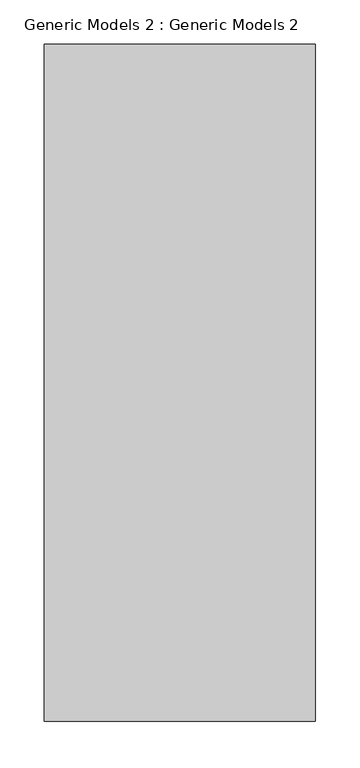
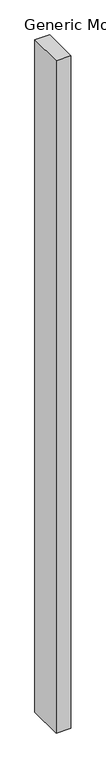
"""IFC4 building model written with IfcOpenShell, lengths in millimetres: proxy geometry, Generic Models 2 : Generic Models 2."""

from ifc_helpers import new_model, si_unit, frame, origin, place, context, project, spatial, polyline, outline, extrude, source, transform, mapped, element, save


def generic_models_2_generic_models_2_fd6437b6(model_context):
    return source(origin(), model_context, "Body", "SweptSolid", [
        extrude(outline(polyline([(13598.5361222, -384.9902311), (13598.5361222, 377.0097689), (13903.3361222, 377.0097689), (13903.3361222, -384.9902311), (13598.5361222, -384.9902311)])), frame((0.0, 0.0, 3840.2215532), z_axis=(0.0, 0.0, 1.0), x_axis=(1.0, 0.0, 0.0)), (0.0, 0.0, 1.0), 14782.8),
    ])


if __name__ == "__main__":
    model = new_model("IFC4")
    model_context = context("Model", 3, world=origin())
    ifc_project = project(units=[si_unit("LENGTHUNIT", "METRE", prefix="MILLI")], contexts=[model_context])
    site = spatial("IfcSite", under=ifc_project)
    building = spatial("IfcBuilding", under=site)
    placement = place(None, origin())
    generic_models_2_generic_models_2_shape = generic_models_2_generic_models_2_fd6437b6(model_context)
    element("IfcBuildingElementProxy", 1, Name="Generic Models 2 : Generic Models 2", ObjectType="Generic Models 2 : Generic Models 2", at=placement, inside=building, context=model_context, shape_type="MappedRepresentation", body=[
        mapped(generic_models_2_generic_models_2_shape, transform((0.0, 0.0, 0.0), x_axis=(1.0, 0.0, 0.0), y_axis=(0.0, 1.0, 0.0), z_axis=(0.0, 0.0, 1.0))),
    ])
    save(model, "model.ifc")
